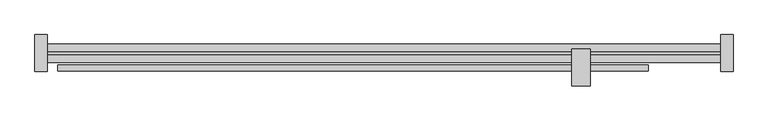
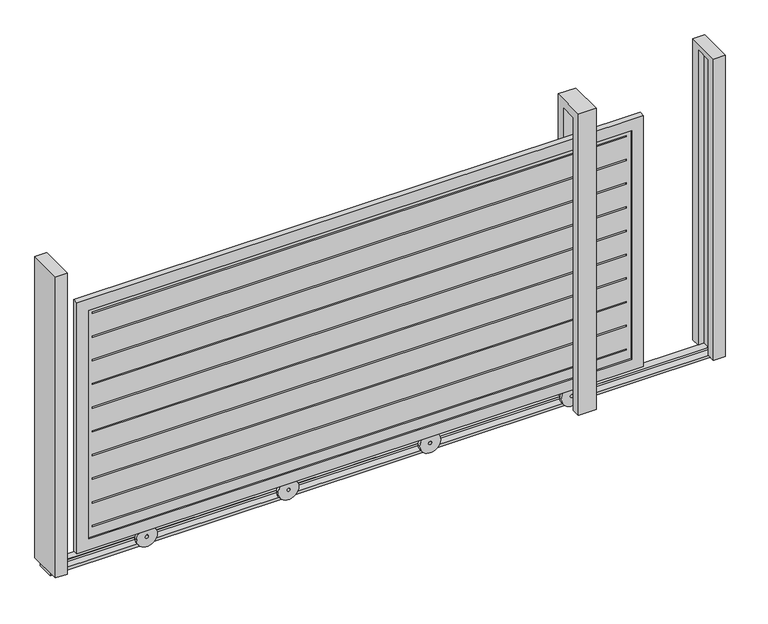
"""IFC4 building model written with IfcOpenShell, lengths in millimetres: geographic element geometry."""

from ifc_helpers import new_model, si_unit, point, frame, frame_2d, origin, place, context, project, spatial, polyline, circle_curve, trimmed, segment, composite_curve, outline, extrude, faceted_brep, source, transform, mapped, element, save


def geographic_element_11039c17(model_context):
    return source(origin(), model_context, "Body", "SolidModel", [
        faceted_brep([(2832.1, 152.4, 0.0), (2882.9, 152.4, 0.0), (2882.9, 0.0, 0.0), (2832.1, 0.0, 0.0), (2832.1, 38.1, 0.0), (2857.5, 38.1, 0.0), (2857.5, 114.3, 0.0), (2832.1, 114.3, 0.0), (2857.5, 114.3, 1346.2), (2832.1, 114.3, 1346.2), (2857.5, 38.1, 1346.2), (2832.1, 38.1, 1346.2), (2832.1, 0.0, 1371.6), (2882.9, 0.0, 1371.6), (2882.9, 152.4, 1371.6), (2832.1, 152.4, 1371.6)], [[[0, 1, 2, 3, 4, 5, 6, 7]], [[6, 8, 9, 7]], [[5, 10, 8, 6]], [[4, 11, 10, 5]], [[12, 3, 2, 13]], [[13, 2, 1, 14]], [[14, 1, 0, 15]], [[11, 4, 3, 12, 15, 0, 7, 9]], [[9, 8, 10, 11]], [[12, 13, 14, 15]]]),
        extrude(outline(composite_curve([segment(trimmed(circle_curve(frame_2d((43.1280612, 399.0102832)), 44.45), [point((43.1280612, 354.5602832))], [point((43.1280612, 443.4602832))], False, "CARTESIAN"), True, "CONTINUOUS"), segment(trimmed(circle_curve(frame_2d((43.1280612, 399.0102832)), 44.45), [point((43.1280612, 443.4602832))], [point((43.1280612, 354.5602832))], False, "CARTESIAN"), True, "CONTINUOUS")], self_intersect=False), holes=[composite_curve([segment(trimmed(circle_curve(frame_2d((43.1280612, 399.0102832)), 6.35), [point((43.1280612, 392.6602832))], [point((43.1280612, 405.3602832))], True, "CARTESIAN"), True, "CONTINUOUS"), segment(trimmed(circle_curve(frame_2d((43.1280612, 399.0102832)), 6.35), [point((43.1280612, 405.3602832))], [point((43.1280612, 392.6602832))], True, "CARTESIAN"), True, "CONTINUOUS")], self_intersect=False)]), frame((0.0, 8.6127422, 0.0), z_axis=(0.0, 1.0, 0.0), x_axis=(0.0, 0.0, 1.0)), (0.0, 0.0, 1.0), 12.7),
        extrude(outline(composite_curve([segment(trimmed(circle_curve(frame_2d((43.1280612, 1618.2102832)), 44.45), [point((43.1280612, 1573.7602832))], [point((43.1280612, 1662.6602832))], False, "CARTESIAN"), True, "CONTINUOUS"), segment(trimmed(circle_curve(frame_2d((43.1280612, 1618.2102832)), 44.45), [point((43.1280612, 1662.6602832))], [point((43.1280612, 1573.7602832))], False, "CARTESIAN"), True, "CONTINUOUS")], self_intersect=False), holes=[composite_curve([segment(trimmed(circle_curve(frame_2d((43.1280612, 1618.2102832)), 6.35), [point((43.1280612, 1611.8602832))], [point((43.1280612, 1624.5602832))], True, "CARTESIAN"), True, "CONTINUOUS"), segment(trimmed(circle_curve(frame_2d((43.1280612, 1618.2102832)), 6.35), [point((43.1280612, 1624.5602832))], [point((43.1280612, 1611.8602832))], True, "CARTESIAN"), True, "CONTINUOUS")], self_intersect=False)]), frame((0.0, 8.6127422, 0.0), z_axis=(0.0, 1.0, 0.0), x_axis=(0.0, 0.0, 1.0)), (0.0, 0.0, 1.0), 12.7),
        extrude(outline(composite_curve([segment(trimmed(circle_curve(frame_2d((43.1280612, 2227.8102832)), 44.45), [point((43.1280612, 2183.3602832))], [point((43.1280612, 2272.2602832))], False, "CARTESIAN"), True, "CONTINUOUS"), segment(trimmed(circle_curve(frame_2d((43.1280612, 2227.8102832)), 44.45), [point((43.1280612, 2272.2602832))], [point((43.1280612, 2183.3602832))], False, "CARTESIAN"), True, "CONTINUOUS")], self_intersect=False), holes=[composite_curve([segment(trimmed(circle_curve(frame_2d((43.1280612, 2227.8102832)), 6.35), [point((43.1280612, 2221.4602832))], [point((43.1280612, 2234.1602832))], True, "CARTESIAN"), True, "CONTINUOUS"), segment(trimmed(circle_curve(frame_2d((43.1280612, 2227.8102832)), 6.35), [point((43.1280612, 2234.1602832))], [point((43.1280612, 2221.4602832))], True, "CARTESIAN"), True, "CONTINUOUS")], self_intersect=False)]), frame((0.0, 8.6127422, 0.0), z_axis=(0.0, 1.0, 0.0), x_axis=(0.0, 0.0, 1.0)), (0.0, 0.0, 1.0), 12.7),
        extrude(outline(composite_curve([segment(trimmed(circle_curve(frame_2d((43.1280612, 1008.6102832)), 44.45), [point((43.1280612, 964.1602832))], [point((43.1280612, 1053.0602832))], False, "CARTESIAN"), True, "CONTINUOUS"), segment(trimmed(circle_curve(frame_2d((43.1280612, 1008.6102832)), 44.45), [point((43.1280612, 1053.0602832))], [point((43.1280612, 964.1602832))], False, "CARTESIAN"), True, "CONTINUOUS")], self_intersect=False), holes=[composite_curve([segment(trimmed(circle_curve(frame_2d((43.1280612, 1008.6102832)), 6.35), [point((43.1280612, 1002.2602832))], [point((43.1280612, 1014.9602832))], True, "CARTESIAN"), True, "CONTINUOUS"), segment(trimmed(circle_curve(frame_2d((43.1280612, 1008.6102832)), 6.35), [point((43.1280612, 1014.9602832))], [point((43.1280612, 1002.2602832))], True, "CARTESIAN"), True, "CONTINUOUS")], self_intersect=False)]), frame((0.0, 8.6127422, 0.0), z_axis=(0.0, 1.0, 0.0), x_axis=(0.0, 0.0, 1.0)), (0.0, 0.0, 1.0), 12.7),
        extrude(outline(polyline([(1217.8780612, 2532.6102832), (1217.8780612, 94.2102832), (74.8780612, 94.2102832), (74.8780612, 2532.6102832), (1217.8780612, 2532.6102832)]), holes=[polyline([(1167.0780612, 145.0102832), (1167.0780612, 2481.8102832), (125.6780612, 2481.8102832), (125.6780612, 145.0102832), (1167.0780612, 145.0102832)])]), frame((0.0, 2.2627422, 0.0), z_axis=(0.0, 1.0, 0.0), x_axis=(0.0, 0.0, 1.0)), (0.0, 0.0, 1.0), 25.4),
        extrude(outline(polyline([(1173.4280612, 2488.1602832), (1173.4280612, 138.6602832), (119.3280612, 138.6602832), (119.3280612, 2488.1602832), (1173.4280612, 2488.1602832)]), holes=[polyline([(1148.0280612, 164.0602832), (1148.0280612, 2462.7602832), (1141.6780612, 2462.7602832), (1141.6780612, 164.0602832), (1148.0280612, 164.0602832)]), polyline([(1040.0780612, 164.0602832), (1040.0780612, 2462.7602832), (1033.7280612, 2462.7602832), (1033.7280612, 164.0602832), (1040.0780612, 164.0602832)]), polyline([(932.1280612, 164.0602832), (932.1280612, 2462.7602832), (925.7780612, 2462.7602832), (925.7780612, 164.0602832), (932.1280612, 164.0602832)]), polyline([(824.1780612, 164.0602832), (824.1780612, 2462.7602832), (817.8280612, 2462.7602832), (817.8280612, 164.0602832), (824.1780612, 164.0602832)]), polyline([(716.2280612, 164.0602832), (716.2280612, 2462.7602832), (709.8780612, 2462.7602832), (709.8780612, 164.0602832), (716.2280612, 164.0602832)]), polyline([(608.2780612, 164.0602832), (608.2780612, 2462.7602832), (601.9280612, 2462.7602832), (601.9280612, 164.0602832), (608.2780612, 164.0602832)]), polyline([(500.3280612, 164.0602832), (500.3280612, 2462.7602832), (493.9780612, 2462.7602832), (493.9780612, 164.0602832), (500.3280612, 164.0602832)]), polyline([(392.3780612, 164.0602832), (392.3780612, 2462.7602832), (386.0280612, 2462.7602832), (386.0280612, 164.0602832), (392.3780612, 164.0602832)]), polyline([(284.4280612, 164.0602832), (284.4280612, 2462.7602832), (278.0780612, 2462.7602832), (278.0780612, 164.0602832), (284.4280612, 164.0602832)]), polyline([(176.4780612, 164.0602832), (176.4780612, 2462.7602832), (170.1280612, 2462.7602832), (170.1280612, 164.0602832), (176.4780612, 164.0602832)])]), frame((0.0, 8.6127422, 0.0), z_axis=(0.0, 1.0, 0.0), x_axis=(0.0, 0.0, 1.0)), (0.0, 0.0, 1.0), 12.7),
        extrude(outline(polyline([(93.4983181, 1371.6), (93.4983181, 0.0), (55.3983181, 0.0), (55.3983181, 1333.5), (-20.8016819, 1333.5), (-20.8016819, 0.0), (-58.9016819, 0.0), (-58.9016819, 1371.6), (93.4983181, 1371.6)])), frame((2217.5186928, 0.0, 0.0), z_axis=(1.0, 0.0, 0.0), x_axis=(0.0, 1.0, 0.0)), (0.0, 0.0, 1.0), 76.2),
        faceted_brep([(50.8, 152.4, 0.0), (50.8, 114.3, 0.0), (25.4, 114.3, 0.0), (25.4, 38.1, 0.0), (50.8, 38.1, 0.0), (50.8, 0.0, 0.0), (0.0, 0.0, 0.0), (0.0, 152.4, 0.0), (50.8, 114.3, 1346.2), (25.4, 114.3, 1346.2), (25.4, 38.1, 1346.2), (50.8, 38.1, 1346.2), (50.8, 0.0, 1371.6), (0.0, 0.0, 1371.6), (0.0, 152.4, 1371.6), (50.8, 152.4, 1371.6)], [[[0, 1, 2, 3, 4, 5, 6, 7]], [[2, 1, 8, 9]], [[3, 2, 9, 10]], [[4, 3, 10, 11]], [[12, 13, 6, 5]], [[13, 14, 7, 6]], [[14, 15, 0, 7]], [[11, 8, 1, 0, 15, 12, 5, 4]], [[8, 11, 10, 9]], [[12, 15, 14, 13]]]),
        extrude(outline(polyline([(83.3319524, 0.0), (114.3, 0.0), (114.3, -12.7), (38.1, -12.7), (38.1, 0.0), (68.8793004, 0.0), (68.8793004, -1.3219388), (83.3319524, -1.3219388), (83.3319524, 0.0)])), frame((0.0, 0.0, 0.0), z_axis=(1.0, 0.0, 0.0), x_axis=(0.0, 1.0, 0.0)), (0.0, 0.0, 1.0), 2857.5),
    ])


if __name__ == "__main__":
    model = new_model("IFC4")
    model_context = context("Model", 3, world=origin())
    ifc_project = project(units=[si_unit("LENGTHUNIT", "METRE", prefix="MILLI")], contexts=[model_context])
    site = spatial("IfcSite", under=ifc_project)
    building = spatial("IfcBuilding", under=site)
    placement = place(None, origin())
    geographic_element_shape = geographic_element_11039c17(model_context)
    element("IfcGeographicElement", 1, at=placement, inside=building, context=model_context, shape_type="MappedRepresentation", body=[
        mapped(geographic_element_shape, transform((0.0, 0.0, 0.0), x_axis=(1.0, 0.0, 0.0), y_axis=(0.0, 1.0, 0.0), z_axis=(0.0, 0.0, 1.0))),
    ])
    save(model, "model.ifc")

# Revit data of these elements
# Type
#   channel width = 16' - 0"
#   Width = 8' - 0"
#   Gate open = 2' - 0"
#   stopper material = aluminium dark grey
#   panel material = wood panel
# Element 1 (IfcGeographicElement)
#   Materials on its faces: "wood panel", "aluminium dark grey", "black metal"
# Materials
#   "aluminium dark grey": class "Generic", colour RGB 85 85 85, transparency 0, Cost = 0
#   "wood panel": class "Generic", colour RGB 128 64 0, transparency 0, Cost = 0
#   "black metal": class "Generic", colour RGB 120 120 120, transparency 0, Cost = 0
